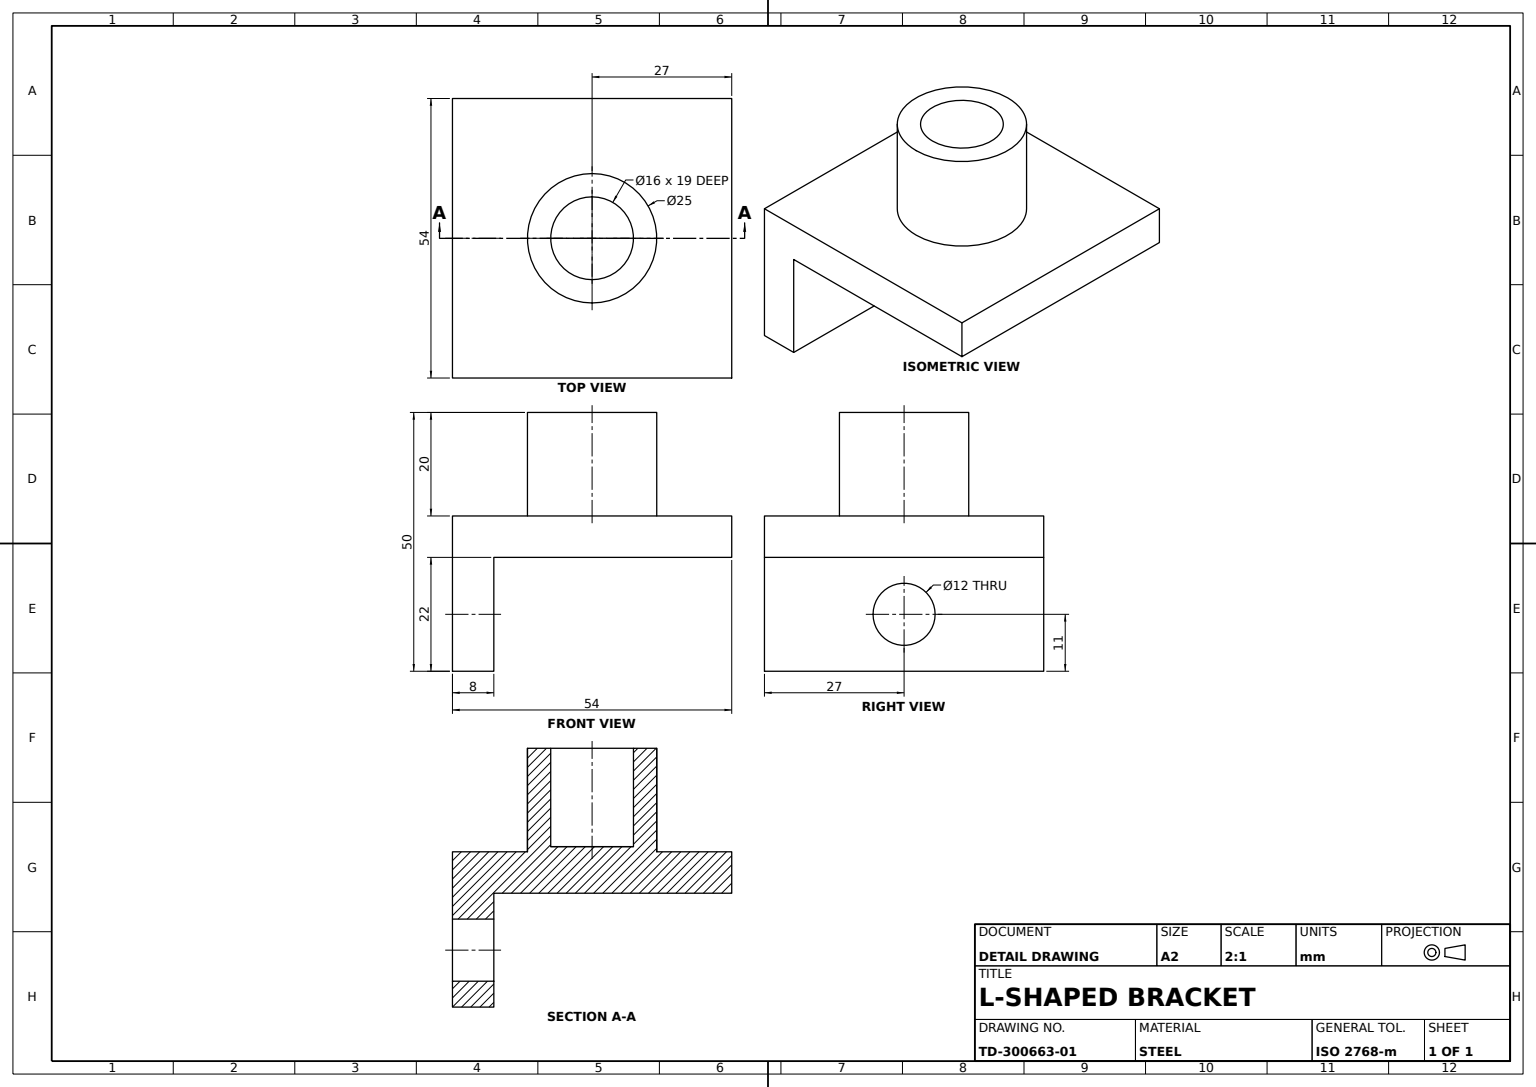
SolidWorks part; units mm, degrees
material "Plain Carbon Steel"
ref_plane "Front Plane" through (0, 0, 0) normal (0, 0, 1) x (1, 0, 0)
ref_plane "Top Plane" through (0, 0, 0) normal (0, 1, 0) x (1, 0, 0)
ref_plane "Right Plane" through (0, 0, 0) normal (1, 0, 0) x (0, 0, -1)
sketch "Bracket Profile Sketch" plane through (0, 0, 0) normal (0, 0, 1) x (1, 0, 0)
  line L0 (0, 0) -> (0, 30)
  line L1 (0, 30) -> (54, 30)
  line L2 (54, 30) -> (54, 22)
  line L3 (54, 22) -> (8, 22)
  line L4 (8, 22) -> (8, 0)
  line L5 (8, 0) -> (0, 0)
  dimension "D1" = 8
  dimension "D2" = 54
  dimension "D3" = 22
extrude "Bracket Body" add sketch "Bracket Profile Sketch" along normal blind 54
sketch "Boss Sketch" plane through (0, 30, 0) normal (0, 1, 0) x (1, 0, 0)
  line L0 (0, -54) -> (0, 0) construction
  line L1 (54, 0) -> (0, 0) construction
  circle A0 centre (27, -27) radius 12.5
  dimension "D1" = 25
  dimension "D3" = 25
  dimension "D2" = 27
  dimension "D4" = 27
extrude "Boss Ø25" add sketch "Boss Sketch" along normal blind 20
sketch "Bore Sketch" plane through (0, 50, 0) normal (0, 1, 0) x (1, 0, 0)
  circle A0 centre (27, -27) radius 8
  dimension "D1" = 16
  dimension "D2" = 16
extrude "Bore Ø16" cut sketch "Bore Sketch" against normal blind 19
sketch "Hole Sketch" plane through (8, 0, 0) normal (1, 0, 0) x (0, 0, -1)
  line L0 (0, 0) -> (0, 22) construction
  line L1 (-54, 22) -> (0, 22) construction
  circle A0 centre (-27, 11) radius 6
  dimension "D1" = 12
  dimension "D2" = 12
  dimension "D3" = 27
  dimension "D4" = 11
extrude "Hole Ø12" cut sketch "Hole Sketch" against normal blind 8
